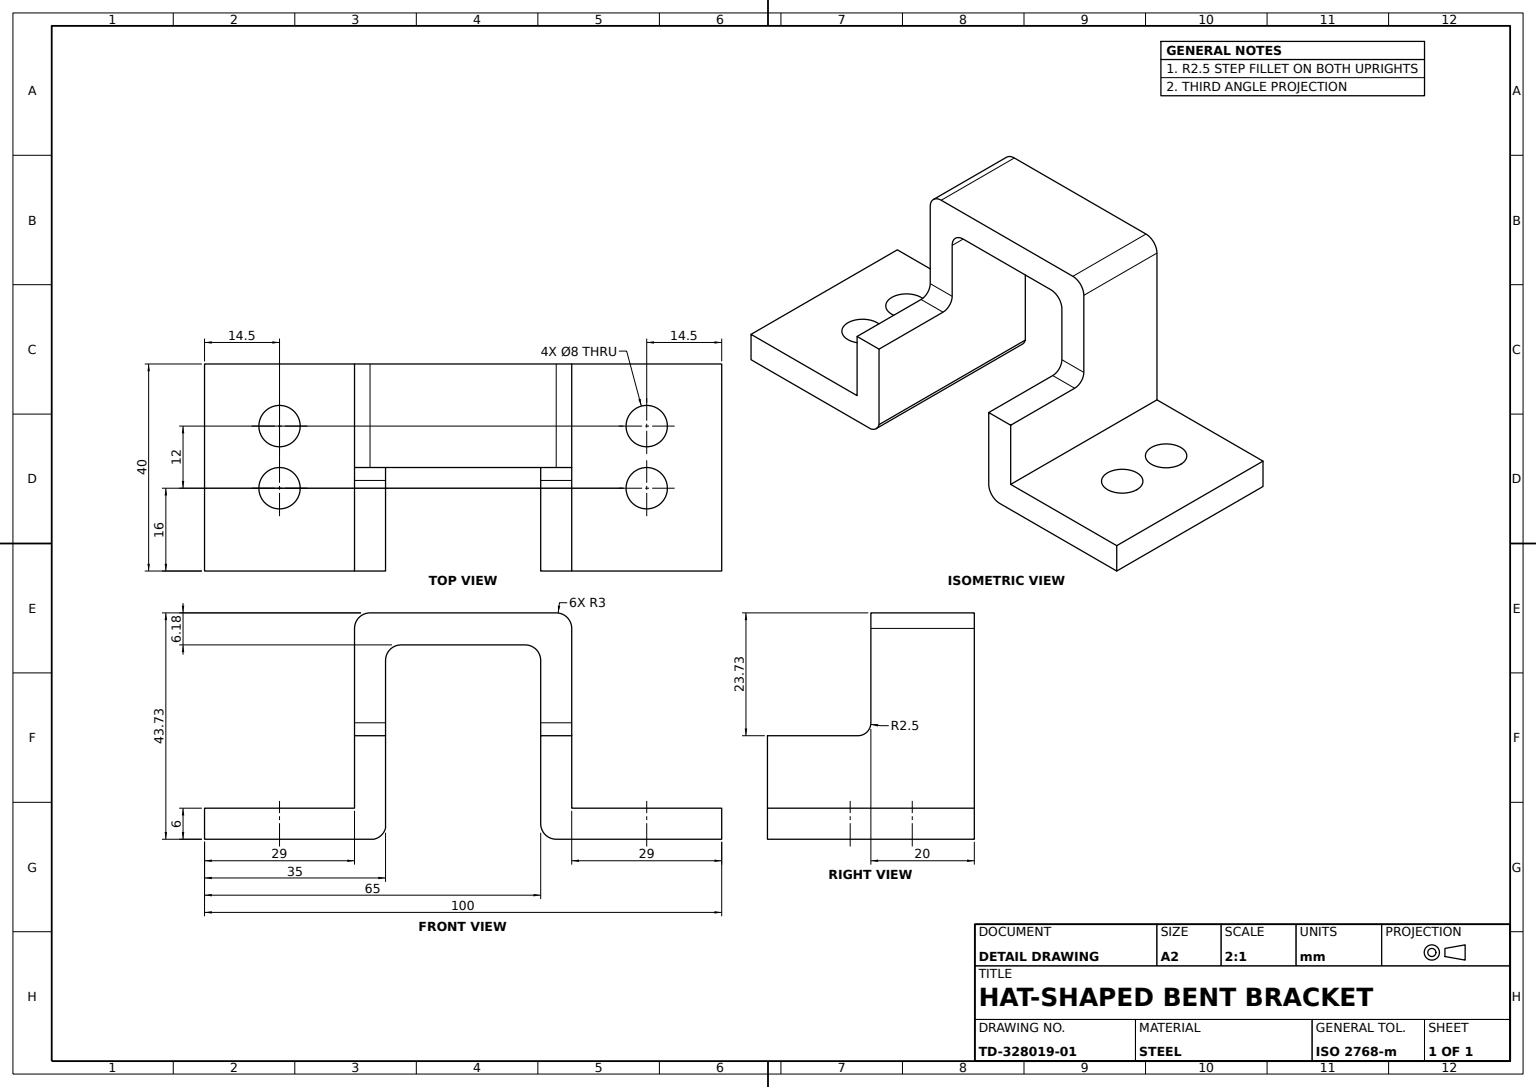
SolidWorks part; units mm, degrees
material "Plain Carbon Steel"
ref_plane "Front Plane" through (0, 0, 0) normal (0, 0, 1) x (1, 0, 0)
ref_plane "Top Plane" through (0, 0, 0) normal (0, 1, 0) x (1, 0, 0)
ref_plane "Right Plane" through (0, 0, 0) normal (1, 0, 0) x (0, 0, -1)
sketch "Bracket Profile Sketch" plane through (0, 0, 0) normal (0, 0, 1) x (1, 0, 0)
  line L1 (30, 0) -> (65, 0)
  line L2 (65, 0) -> (65, 6)
  line L3 (65, 6) -> (36, 6)
  line L4 (36, 6) -> (36, 40.7317)
  line L8 (-35, 6) -> (-35, 0)
  line L9 (-35, 0) -> (0, 0)
  line L11 (15.5197, 0.5517) -> (15.5197, 43.7317) construction
  line L12 (33, 43.7317) -> (-3, 43.7317)
  line L13 (-6, 40.7317) -> (-6, 6)
  line L14 (-6, 6) -> (-35, 6)
  line L15 (0, 0) -> (0, 34.5478)
  line L16 (3, 37.5478) -> (27, 37.5478)
  line L17 (30, 34.5478) -> (30, 0)
  arc A1 (36, 40.7317) -> (33, 43.7317) centre (33, 40.7317) ccw
  arc A2 (-3, 43.7317) -> (-6, 40.7317) centre (-3, 40.7317) ccw
  arc A3 (30, 34.5478) -> (27, 37.5478) centre (27, 34.5478) ccw
  arc A4 (3, 37.5478) -> (0, 34.5478) centre (3, 34.5478) ccw
  dimension "D1" = 6
  dimension "D8" = 3
  dimension "D9" = 3
  dimension "D10" = 43.8469
  dimension "D11" = 3
  dimension "D13" = 3
  dimension "D2" = 6
  dimension "D3" = 6
  dimension "D4" = 6
  dimension "D5" = 30
  dimension "D6" = 65
  dimension "D7" = 35
  dimension "D12" = 20.4803
  dimension "D14" = 43.7317
extrude "Bracket Body 40mm" add sketch "Bracket Profile Sketch" along normal mid plane 40
sketch "Relief Cut Sketch" plane through (0, 0, 0) normal (0, 0, 1) x (1, 0, 0)
  line L0 (0, 0) -> (0, 20)
  line L1 (0, 0) -> (0, 34.5478) construction
  line L2 (0, 20) -> (0, 34.5478)
  line L3 (3, 37.5478) -> (27, 37.5478)
  line L4 (30, 34.5478) -> (30, 20)
  line L5 (30, 34.5478) -> (30, 0) construction
  line L6 (30, 20) -> (36, 20)
  line L7 (36, 6) -> (36, 40.7317) construction
  line L8 (36, 20) -> (36, 40.7317)
  line L9 (33, 43.7317) -> (-3, 43.7317)
  line L10 (-6, 40.7317) -> (-6, 20)
  line L11 (-6, 40.7317) -> (-6, 6) construction
  line L12 (-6, 20) -> (0, 20)
  arc A0 (0, 34.5478) -> (3, 37.5478) centre (3, 34.5478) cw
  arc A1 (27, 37.5478) -> (30, 34.5478) centre (27, 34.5478) cw
  arc A2 (36, 40.7317) -> (33, 43.7317) centre (33, 40.7317) ccw
  arc A3 (-3, 43.7317) -> (-6, 40.7317) centre (-3, 40.7317) ccw
  dimension "D1" = 23.7317
extrude "Stepped Relief Cut 28mm" cut sketch "Relief Cut Sketch" along normal blind 28 contours L9 A3 L10 L12 L2 A0 L3 A1 L4 L6 L8 A2
sketch "Corner Round Cut A Sketch" plane through (0, 0, 20) normal (0, 0, 1) x (1, 0, 0)
  line L0 (0, 0) -> (0, 20) construction
  line L1 (-35, 0) -> (0, 0) construction
  line L2 (0, 2.1404) -> (0, 0)
  line L3 (0, 0) -> (-2.2529, 0)
  line L4 (-6, 20) -> (-6, 6) construction
  arc A0 (0, 2.1404) -> (-2.2529, 0) centre (-2.894, 2.9307) cw
  dimension "D1" = 3
  dimension "D2" = 3.106
  dimension "D3" = 3.7471
extrude "Corner Round Cut A R3" cut sketch "Corner Round Cut A Sketch" against normal through all
sketch "Corner Round Cut B Sketch" plane through (0, 0, 0) normal (0, 0, 1) x (1, 0, 0)
  line L0 (30, 0) -> (30, 3)
  line L1 (30, 20) -> (30, 0) construction
  line L2 (30, 0) -> (33, 0)
  line L3 (30, 0) -> (65, 0) construction
  arc A0 (30, 3) -> (33, 0) centre (33, 3) ccw
  dimension "D1" = 3
extrude "Corner Round Cut B R3" cut sketch "Corner Round Cut B Sketch" against normal through all both and the other way through all
sketch "Corner Fill Boss A Sketch" plane through (-6, 0, 0) normal (-1, 0, 0) x (0, 0, 1)
  line L0 (0, 20) -> (0, 22.5)
  line L1 (0, 40.7317) -> (0, 20) construction
  line L2 (0, 20) -> (2.5, 20)
  line L3 (20, 20) -> (0, 20) construction
  arc A0 (0, 22.5) -> (2.5, 20) centre (2.5, 22.5) ccw
  dimension "D1" = 2.5
extrude "Corner Fill Boss A 6mm" add sketch "Corner Fill Boss A Sketch" against normal blind 6
sketch "Corner Fill Boss B Sketch" plane through (36, 0, 0) normal (1, 0, 0) x (0, 0, -1)
  line L0 (0, 22.5) -> (0, 20)
  line L1 (0, 20) -> (-2.5, 20)
  arc A0 (-2.5, 20) -> (0, 22.5) centre (-2.5, 22.5) ccw
extrude "Corner Fill Boss B 6mm" add sketch "Corner Fill Boss B Sketch" against normal blind 6
sketch "Mounting Holes Sketch" plane through (0, 6, 0) normal (0, 1, 0) x (1, 0, 0)
  line L0 (50.5, -20) -> (50.5, -4) construction
  line L1 (65, -20) -> (36, -20) construction
  line L2 (50.5, -4) -> (50.5, 8) construction
  line L4 (15, 20) -> (15, -20) construction
  line L5 (33, 20) -> (-3, 20) construction
  circle A0 centre (50.5, -4) radius 4
  circle A1 centre (50.5, 8) radius 4
  circle A2 centre (-20.5, -4) radius 4
  circle A3 centre (-20.5, 8) radius 4
  dimension "D1" = 16
  dimension "D3" = 8
  dimension "D4" = 8
  dimension "D2" = 12
extrude "Flange Mounting Holes" cut sketch "Mounting Holes Sketch" against normal through all
